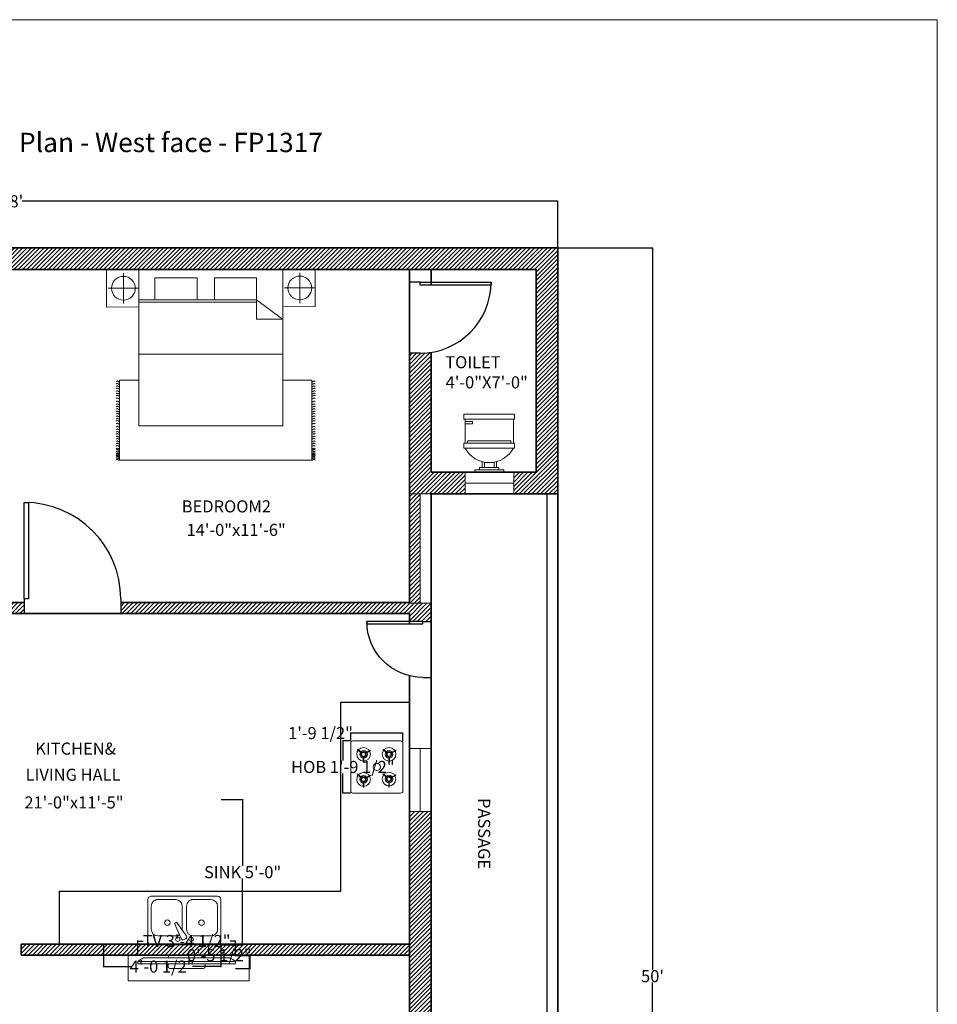
# Model space of a CAD drawing. Units: inches. Extents: x 2202345 to 2203065, y -970921 to -970107.
# Tile 5 of 5: x 2202685 to 2203065, y -970515 to -970107. Entities that reach past the tile are written whole.
import ezdxf

# ---------------------------------------------------------------- set-up
doc = ezdxf.new("R2010")
doc.units = ezdxf.units.IN
doc.header["$MEASUREMENT"] = 0
doc.linetypes.add('HIDDEN', pattern=[0.375, 0.25, -0.125])
doc.layers.get('0').update_dxf_attribs({"color": 13})
for name, color, linetype, lineweight in [('A-ANNO-DIMS', 2, 'Continuous', 18), ('A-ANNO-TEXT', 7, 'Continuous', 25), ('A-ANNO-TTLB', 7, 'HIDDEN', 18), ('A-AREA-IDEN', 7, 'Continuous', 18), ('A-EQPM', 8, 'Continuous', 18), ('A-FLOR-CASE', 252, 'Continuous', 25), ('A-WALL-PATT', 8, 'Continuous', 13), ('C-PROP', 7, 'Continuous', 25), ('doors', 252, 'Continuous', 25), ('furniture', 250, 'Continuous', 18), ('PLUMBING FIXTURES', 8, 'Continuous', 18), ('walls', 252, 'Continuous', 35), ('windows', 173, 'Continuous', 18)]:
    doc.layers.add(name, color=color, linetype=linetype, lineweight=lineweight)
doc.styles.add('ATT', font='TXT')
doc.styles.get("Standard").update_dxf_attribs({"font": 'arial.ttf'})
doc.dimstyles.get("Standard").update_dxf_attribs({"dimtxt": 5, "dimasz": 0.18, "dimexe": 0.18, "dimexo": 0.0625, "dimgap": 0.09, "dimtad": 0, "dimtih": 1, "dimtoh": 1, "dimzin": 0, "dimdsep": 46, "dimlunit": 3, "dimtxsty": 'Standard', "dimcen": 0.09, "dimadec": 0, "dimazin": 0, "dimtfac": 1, "dimtofl": 0, "dimtmove": 0, "dimatfit": 3, "dimfxl": 1, "dimtolj": 1, "dimtzin": 0, "dimarcsym": 0})
pattern_1 = [(45, (0, 0), (-0.8838834765, 0.8838834765), [])]

# ---------------------------------------------------------------- blocks, each defined once
blk = doc.blocks.new('4bstove')
at = {"layer": 'furniture'}
for p, q in [((1452.73, 1446.21), (1452.73, 1448.61)), ((1452.98, 1446.22), (1452.98, 1448.61)), ((1464.44, 1446.34), (1464.44, 1448.73)), ((1464.69, 1446.34), (1464.69, 1448.73)), ((1451.74, 1444.45), (1449.67, 1443.25)), ((1451.87, 1444.23), (1449.79, 1443.04)), ((1453.75, 1444.08), (1455.58, 1442.54)), ((1453.91, 1444.27), (1455.74, 1442.73)), ((1463.45, 1444.58), (1461.38, 1443.38)), ((1463.57, 1444.36), (1461.5, 1443.17)), ((1465.46, 1444.21), (1467.29, 1442.67)), ((1465.62, 1444.4), (1467.45, 1442.86)), ((1452.69, 1434.81), (1452.69, 1437.2)), ((1452.94, 1434.81), (1452.94, 1437.2)), ((1464.44, 1434.81), (1464.44, 1437.2)), ((1464.69, 1434.81), (1464.69, 1437.2)), ((1451.7, 1433.04), (1449.63, 1431.85)), ((1451.82, 1432.83), (1449.75, 1431.63)), ((1453.71, 1432.67), (1455.54, 1431.13)), ((1453.87, 1432.86), (1455.7, 1431.33)), ((1463.45, 1433.04), (1461.38, 1431.85)), ((1463.57, 1432.83), (1461.5, 1431.63)), ((1465.46, 1432.67), (1467.29, 1431.13)), ((1465.62, 1432.86), (1467.45, 1431.33))]:
    blk.add_line(p, q, dxfattribs=at)
for points in [[(1447.5, 1427.38), (1469.5, 1427.38, 0.414214), (1470.5, 1428.38), (1470.5, 1450.38, 0.414214), (1469.5, 1451.38), (1447.5, 1451.38, 0.414214), (1446.5, 1450.38), (1446.5, 1428.38, 0.414214)], [(1453.75, 1444.97, 1), (1452, 1444.97, 1)], [(1465.46, 1445.1, 1), (1463.71, 1445.1, 1)], [(1453.71, 1433.56, 1), (1451.96, 1433.56, 1)], [(1465.46, 1433.56, 1), (1463.71, 1433.56, 1)]]:
    blk.add_lwpolyline(points, format="xyb", close=True, dxfattribs=at)
for points in [[(1454.12, 1444.97, 1), (1451.62, 1444.97, 1), (1454.12, 1444.97, 1)], [(1465.83, 1445.1, 1), (1463.33, 1445.1, 1), (1465.83, 1445.1, 1)], [(1454.08, 1433.56, 1), (1451.58, 1433.56, 1), (1454.08, 1433.56, 1)], [(1465.83, 1433.56, 1), (1463.33, 1433.56, 1), (1465.83, 1433.56, 1)]]:
    blk.add_lwpolyline(points, format="xyb", dxfattribs=at)
for centre, radius in [((1452.87, 1444.97), 3.14), ((1452.87, 1444.97), 1.75), ((1464.58, 1445.1), 3.14), ((1464.58, 1445.1), 1.75), ((1452.83, 1433.56), 3.14), ((1458.5, 1439.38), 1.67), ((1464.58, 1433.56), 3.14), ((1452.83, 1433.56), 1.75), ((1464.58, 1433.56), 1.75)]:
    blk.add_circle(centre, radius, dxfattribs=at)
for centre, start, end in [((1452.87, 1444.97), 88.2645, 92.2039), ((1464.58, 1445.1), 88.2645, 92.2039), ((1452.87, 1444.97), 208.188, 212.1274), ((1452.87, 1444.97), 318.1018, 322.0412), ((1464.58, 1445.1), 208.188, 212.1274), ((1464.58, 1445.1), 318.1018, 322.0412), ((1452.83, 1433.56), 88.2645, 92.2039), ((1464.58, 1433.56), 88.2645, 92.2039)]:
    blk.add_arc(centre, 3.64, start, end, dxfattribs=at)
blk = doc.blocks.new('15PSNK10')
at = {"color": 0, "linetype": 'ByBlock'}
for p, q in [((0, 15), (0, -15)), ((20.5, 16.5), (1.5, 16.5)), ((7, 15), (17.5, 15)), ((22, -15), (22, 15)), ((4, 4), (4, 12)), ((20.5, 12), (20.5, 4)), ((2.37, -0.1), (2.77, 0.6)), ((10.18, -3.57), (4.27, 0.87)), ((17.5, 1), (7, 1)), ((2.88, -1.54), (9.68, -4.43)), ((4, -12), (4, -4)), ((7.04, -1), (17.5, -1)), ((9.68, -4.43), (10.18, -3.57)), ((20.5, -4), (20.5, -12)), ((1.5, -16.5), (20.5, -16.5)), ((17.5, -15), (7, -15))]:
    blk.add_line(p, q, dxfattribs=at)
for centre, radius in [((10, 7.75), 1.25), ((2.5, 3), 1), ((2.5, -3), 1), ((10, -7.75), 1.25)]:
    blk.add_circle(centre, radius, dxfattribs=at)
for centre, radius, start, end in [((1.5, 15), 1.5, 90, 180), ((7, 12), 3, 90, 180), ((17.5, 12), 3, 0, 90), ((20.5, 15), 1.5, 0, 90), ((3.63, 0.1), 1, 50.5377, 150), ((7, 4), 3, 180, 270), ((17.5, 4), 3, 270, 0), ((3.23, -0.6), 1, 150, 249.4623), ((7, -4), 3, 146.607, 180), ((17.5, -4), 3, 0, 90), ((7, -12), 3, 180, 270), ((17.5, -12), 3, 270, 0), ((1.5, -15), 1.5, 180, 270), ((20.5, -15), 1.5, 270, 0)]:
    blk.add_arc(centre, radius, start, end, dxfattribs=at)
at = {"color": 0, "linetype": 'ByBlock', "style": 'ATT'}
for tag, p, flags in [('ITEM', (0, -26), 3), ('ROOM_NUMBER', (0, -35), 1)]:
    blk.add_attdef(tag, p, '', height=6, dxfattribs=dict(at, flags=flags))
blk = doc.blocks.new('PLASMA-LARGE')
at = {"layer": 'furniture'}
for p, q in [((-7.26, 0), (7.26, 0)), ((-21, -2.5), (21, -2.5)), ((-21, -2.5), (-21, -3.5)), ((-21, -3.5), (21, -3.5)), ((-18.61, -1), (18.61, -1)), ((-8, -1), (-8, -0.74)), ((-8, -3.5), (-8, -4.76)), ((8, -1), (8, -0.74)), ((8, -3.5), (8, -4.76)), ((21, -2.5), (21, -3.5)), ((-7.26, -5.5), (7.26, -5.5))]:
    blk.add_line(p, q, dxfattribs=at)
for centre, radius, start, end in [((-7.26, -0.74), 0.744, 90, 180), ((7.26, -0.74), 0.744, 0, 90), ((-13.97, -11.05), 11.07, 114.7602, 129.4175), ((13.97, -11.05), 11.07, 50.5825, 65.2398), ((-7.26, -4.76), 0.744, 180, 270), ((7.26, -4.76), 0.744, 270, 0)]:
    blk.add_arc(centre, radius, start, end, dxfattribs=at)
blk = doc.blocks.new('CARPET')
at = {"layer": 'furniture'}
for p, q in [((-51.53, -98.11), (-51.53, -55.12)), ((-51.53, -55.12), (-41.27, -55.12)), ((36, -55.12), (51.55, -55.12)), ((51.55, -55.12), (51.55, -98.11)), ((51.55, -98.11), (-51.53, -98.11))]:
    blk.add_line(p, q, dxfattribs=at)
for points, knots in [([(-53.37, -55.99), (-53.22, -55.8), (-52.9, -55.41), (-52.34, -55.8), (-51.89, -56.08), (-51.65, -55.91), (-51.53, -55.83)], [0, 0, 0, 0, 0.653278, 1.290138, 1.740457, 2.114451, 2.114451, 2.114451, 2.114451]), ([(-53.37, -57.26), (-53.22, -57.07), (-52.9, -56.67), (-52.34, -57.07), (-51.89, -57.35), (-51.65, -57.17), (-51.53, -57.1)], [0, 0, 0, 0, 0.653278, 1.290138, 1.740457, 2.114451, 2.114451, 2.114451, 2.114451]), ([(53.37, -55.99), (53.22, -55.8), (52.9, -55.41), (52.34, -55.8), (51.89, -56.08), (51.65, -55.91), (51.53, -55.83)], [0, 0, 0, 0, 0.653278, 1.290138, 1.740457, 2.114451, 2.114451, 2.114451, 2.114451]), ([(53.37, -57.26), (53.22, -57.07), (52.9, -56.67), (52.34, -57.07), (51.89, -57.35), (51.65, -57.17), (51.53, -57.1)], [0, 0, 0, 0, 0.653278, 1.290138, 1.740457, 2.114451, 2.114451, 2.114451, 2.114451]), ([(-53.37, -58.59), (-53.22, -58.4), (-52.9, -58.01), (-52.34, -58.4), (-51.89, -58.68), (-51.65, -58.5), (-51.53, -58.43)], [0, 0, 0, 0, 0.653278, 1.290138, 1.740457, 2.114451, 2.114451, 2.114451, 2.114451]), ([(-53.37, -59.78), (-53.22, -59.58), (-52.9, -59.19), (-52.34, -59.58), (-51.89, -59.86), (-51.65, -59.69), (-51.53, -59.61)], [0, 0, 0, 0, 0.653278, 1.290138, 1.740457, 2.114451, 2.114451, 2.114451, 2.114451]), ([(-53.37, -61.22), (-53.22, -61.02), (-52.9, -60.63), (-52.34, -61.02), (-51.89, -61.3), (-51.65, -61.13), (-51.53, -61.05)], [0, 0, 0, 0, 0.653278, 1.290138, 1.740457, 2.114451, 2.114451, 2.114451, 2.114451]), ([(-53.37, -62.44), (-53.22, -62.25), (-52.9, -61.86), (-52.34, -62.25), (-51.89, -62.53), (-51.65, -62.36), (-51.53, -62.28)], [0, 0, 0, 0, 0.653278, 1.290138, 1.740457, 2.114451, 2.114451, 2.114451, 2.114451]), ([(-53.37, -63.63), (-53.22, -63.43), (-52.9, -63.04), (-52.34, -63.43), (-51.89, -63.72), (-51.65, -63.54), (-51.53, -63.46)], [0, 0, 0, 0, 0.653278, 1.290138, 1.740457, 2.114451, 2.114451, 2.114451, 2.114451]), ([(53.37, -58.59), (53.22, -58.4), (52.9, -58.01), (52.34, -58.4), (51.89, -58.68), (51.65, -58.5), (51.53, -58.43)], [0, 0, 0, 0, 0.653278, 1.290138, 1.740457, 2.114451, 2.114451, 2.114451, 2.114451]), ([(53.37, -59.78), (53.22, -59.58), (52.9, -59.19), (52.34, -59.58), (51.89, -59.86), (51.65, -59.69), (51.53, -59.61)], [0, 0, 0, 0, 0.653278, 1.290138, 1.740457, 2.114451, 2.114451, 2.114451, 2.114451]), ([(53.37, -61.22), (53.22, -61.02), (52.9, -60.63), (52.34, -61.02), (51.89, -61.3), (51.65, -61.13), (51.53, -61.05)], [0, 0, 0, 0, 0.653278, 1.290138, 1.740457, 2.114451, 2.114451, 2.114451, 2.114451]), ([(53.37, -62.44), (53.22, -62.25), (52.9, -61.86), (52.34, -62.25), (51.89, -62.53), (51.65, -62.36), (51.53, -62.28)], [0, 0, 0, 0, 0.653278, 1.290138, 1.740457, 2.114451, 2.114451, 2.114451, 2.114451]), ([(53.37, -63.63), (53.22, -63.43), (52.9, -63.04), (52.34, -63.43), (51.89, -63.72), (51.65, -63.54), (51.53, -63.46)], [0, 0, 0, 0, 0.653278, 1.290138, 1.740457, 2.114451, 2.114451, 2.114451, 2.114451]), ([(-53.37, -65.07), (-53.22, -64.87), (-52.9, -64.48), (-52.34, -64.87), (-51.89, -65.15), (-51.65, -64.98), (-51.53, -64.9)], [0, 0, 0, 0, 0.653278, 1.290138, 1.740457, 2.114451, 2.114451, 2.114451, 2.114451]), ([(-53.37, -66.76), (-53.22, -66.56), (-52.9, -66.17), (-52.34, -66.56), (-51.89, -66.84), (-51.65, -66.67), (-51.53, -66.59)], [0, 0, 0, 0, 0.653278, 1.290138, 1.740457, 2.114451, 2.114451, 2.114451, 2.114451]), ([(-53.37, -68.2), (-53.22, -68), (-52.9, -67.61), (-52.34, -68), (-51.89, -68.28), (-51.65, -68.11), (-51.53, -68.03)], [0, 0, 0, 0, 0.653278, 1.290138, 1.740457, 2.114451, 2.114451, 2.114451, 2.114451]), ([(53.37, -65.07), (53.22, -64.87), (52.9, -64.48), (52.34, -64.87), (51.89, -65.15), (51.65, -64.98), (51.53, -64.9)], [0, 0, 0, 0, 0.653278, 1.290138, 1.740457, 2.114451, 2.114451, 2.114451, 2.114451]), ([(53.37, -66.76), (53.22, -66.56), (52.9, -66.17), (52.34, -66.56), (51.89, -66.84), (51.65, -66.67), (51.53, -66.59)], [0, 0, 0, 0, 0.653278, 1.290138, 1.740457, 2.114451, 2.114451, 2.114451, 2.114451]), ([(53.37, -68.2), (53.22, -68), (52.9, -67.61), (52.34, -68), (51.89, -68.28), (51.65, -68.11), (51.53, -68.03)], [0, 0, 0, 0, 0.653278, 1.290138, 1.740457, 2.114451, 2.114451, 2.114451, 2.114451]), ([(-53.37, -69.53), (-53.22, -69.33), (-52.9, -68.94), (-52.34, -69.33), (-51.89, -69.61), (-51.65, -69.44), (-51.53, -69.36)], [0, 0, 0, 0, 0.653278, 1.290138, 1.740457, 2.114451, 2.114451, 2.114451, 2.114451]), ([(-53.37, -70.79), (-53.22, -70.6), (-52.9, -70.21), (-52.34, -70.6), (-51.89, -70.88), (-51.65, -70.7), (-51.53, -70.63)], [0, 0, 0, 0, 0.653278, 1.290138, 1.740457, 2.114451, 2.114451, 2.114451, 2.114451]), ([(-53.37, -72.12), (-53.22, -71.93), (-52.9, -71.54), (-52.34, -71.93), (-51.89, -72.21), (-51.65, -72.04), (-51.53, -71.96)], [0, 0, 0, 0, 0.653278, 1.290138, 1.740457, 2.114451, 2.114451, 2.114451, 2.114451]), ([(-53.37, -73.31), (-53.22, -73.11), (-52.9, -72.72), (-52.34, -73.11), (-51.89, -73.4), (-51.65, -73.22), (-51.53, -73.14)], [0, 0, 0, 0, 0.653278, 1.290138, 1.740457, 2.114451, 2.114451, 2.114451, 2.114451]), ([(53.37, -69.53), (53.22, -69.33), (52.9, -68.94), (52.34, -69.33), (51.89, -69.61), (51.65, -69.44), (51.53, -69.36)], [0, 0, 0, 0, 0.653278, 1.290138, 1.740457, 2.114451, 2.114451, 2.114451, 2.114451]), ([(53.37, -70.79), (53.22, -70.6), (52.9, -70.21), (52.34, -70.6), (51.89, -70.88), (51.65, -70.7), (51.53, -70.63)], [0, 0, 0, 0, 0.653278, 1.290138, 1.740457, 2.114451, 2.114451, 2.114451, 2.114451]), ([(53.37, -72.12), (53.22, -71.93), (52.9, -71.54), (52.34, -71.93), (51.89, -72.21), (51.65, -72.04), (51.53, -71.96)], [0, 0, 0, 0, 0.653278, 1.290138, 1.740457, 2.114451, 2.114451, 2.114451, 2.114451]), ([(53.37, -73.31), (53.22, -73.11), (52.9, -72.72), (52.34, -73.11), (51.89, -73.4), (51.65, -73.22), (51.53, -73.14)], [0, 0, 0, 0, 0.653278, 1.290138, 1.740457, 2.114451, 2.114451, 2.114451, 2.114451]), ([(-53.37, -74.75), (-53.22, -74.55), (-52.9, -74.16), (-52.34, -74.55), (-51.89, -74.83), (-51.65, -74.66), (-51.53, -74.58)], [0, 0, 0, 0, 0.653278, 1.290138, 1.740457, 2.114451, 2.114451, 2.114451, 2.114451]), ([(-53.37, -75.98), (-53.22, -75.78), (-52.9, -75.39), (-52.34, -75.78), (-51.89, -76.06), (-51.65, -75.89), (-51.53, -75.81)], [0, 0, 0, 0, 0.653278, 1.290138, 1.740457, 2.114451, 2.114451, 2.114451, 2.114451]), ([(-53.37, -77.16), (-53.22, -76.96), (-52.9, -76.57), (-52.34, -76.96), (-51.89, -77.25), (-51.65, -77.07), (-51.53, -76.99)], [0, 0, 0, 0, 0.653278, 1.290138, 1.740457, 2.114451, 2.114451, 2.114451, 2.114451]), ([(-53.37, -78.6), (-53.22, -78.4), (-52.9, -78.01), (-52.34, -78.4), (-51.89, -78.68), (-51.65, -78.51), (-51.53, -78.43)], [0, 0, 0, 0, 0.653278, 1.290138, 1.740457, 2.114451, 2.114451, 2.114451, 2.114451]), ([(53.37, -74.75), (53.22, -74.55), (52.9, -74.16), (52.34, -74.55), (51.89, -74.83), (51.65, -74.66), (51.53, -74.58)], [0, 0, 0, 0, 0.653278, 1.290138, 1.740457, 2.114451, 2.114451, 2.114451, 2.114451]), ([(53.37, -75.98), (53.22, -75.78), (52.9, -75.39), (52.34, -75.78), (51.89, -76.06), (51.65, -75.89), (51.53, -75.81)], [0, 0, 0, 0, 0.653278, 1.290138, 1.740457, 2.114451, 2.114451, 2.114451, 2.114451]), ([(53.37, -77.16), (53.22, -76.96), (52.9, -76.57), (52.34, -76.96), (51.89, -77.25), (51.65, -77.07), (51.53, -76.99)], [0, 0, 0, 0, 0.653278, 1.290138, 1.740457, 2.114451, 2.114451, 2.114451, 2.114451]), ([(53.37, -78.6), (53.22, -78.4), (52.9, -78.01), (52.34, -78.4), (51.89, -78.68), (51.65, -78.51), (51.53, -78.43)], [0, 0, 0, 0, 0.653278, 1.290138, 1.740457, 2.114451, 2.114451, 2.114451, 2.114451]), ([(-53.37, -80.29), (-53.22, -80.09), (-52.9, -79.7), (-52.34, -80.09), (-51.89, -80.37), (-51.65, -80.2), (-51.53, -80.12)], [0, 0, 0, 0, 0.653278, 1.290138, 1.740457, 2.114451, 2.114451, 2.114451, 2.114451]), ([(-53.37, -81.73), (-53.22, -81.53), (-52.9, -81.14), (-52.34, -81.53), (-51.89, -81.81), (-51.65, -81.64), (-51.53, -81.56)], [0, 0, 0, 0, 0.653278, 1.290138, 1.740457, 2.114451, 2.114451, 2.114451, 2.114451]), ([(-53.37, -83.06), (-53.22, -82.86), (-52.9, -82.47), (-52.34, -82.86), (-51.89, -83.14), (-51.65, -82.97), (-51.53, -82.89)], [0, 0, 0, 0, 0.653278, 1.290138, 1.740457, 2.114451, 2.114451, 2.114451, 2.114451]), ([(-53.37, -84.18), (-53.22, -83.99), (-52.9, -83.6), (-52.34, -83.99), (-51.89, -84.27), (-51.65, -84.09), (-51.53, -84.02)], [0, 0, 0, 0, 0.653278, 1.290138, 1.740457, 2.114451, 2.114451, 2.114451, 2.114451]), ([(53.37, -80.29), (53.22, -80.09), (52.9, -79.7), (52.34, -80.09), (51.89, -80.37), (51.65, -80.2), (51.53, -80.12)], [0, 0, 0, 0, 0.653278, 1.290138, 1.740457, 2.114451, 2.114451, 2.114451, 2.114451]), ([(53.37, -81.73), (53.22, -81.53), (52.9, -81.14), (52.34, -81.53), (51.89, -81.81), (51.65, -81.64), (51.53, -81.56)], [0, 0, 0, 0, 0.653278, 1.290138, 1.740457, 2.114451, 2.114451, 2.114451, 2.114451]), ([(53.37, -83.06), (53.22, -82.86), (52.9, -82.47), (52.34, -82.86), (51.89, -83.14), (51.65, -82.97), (51.53, -82.89)], [0, 0, 0, 0, 0.653278, 1.290138, 1.740457, 2.114451, 2.114451, 2.114451, 2.114451]), ([(53.37, -84.18), (53.22, -83.99), (52.9, -83.6), (52.34, -83.99), (51.89, -84.27), (51.65, -84.09), (51.53, -84.02)], [0, 0, 0, 0, 0.653278, 1.290138, 1.740457, 2.114451, 2.114451, 2.114451, 2.114451]), ([(-53.37, -85.51), (-53.22, -85.32), (-52.9, -84.93), (-52.34, -85.32), (-51.89, -85.6), (-51.65, -85.42), (-51.53, -85.35)], [0, 0, 0, 0, 0.653278, 1.290138, 1.740457, 2.114451, 2.114451, 2.114451, 2.114451]), ([(-53.37, -86.7), (-53.22, -86.5), (-52.9, -86.11), (-52.34, -86.5), (-51.89, -86.78), (-51.65, -86.61), (-51.53, -86.53)], [0, 0, 0, 0, 0.653278, 1.290138, 1.740457, 2.114451, 2.114451, 2.114451, 2.114451]), ([(-53.37, -88.14), (-53.22, -87.94), (-52.9, -87.55), (-52.34, -87.94), (-51.89, -88.22), (-51.65, -88.05), (-51.53, -87.97)], [0, 0, 0, 0, 0.653278, 1.290138, 1.740457, 2.114451, 2.114451, 2.114451, 2.114451]), ([(-53.37, -89.36), (-53.22, -89.17), (-52.9, -88.78), (-52.34, -89.17), (-51.89, -89.45), (-51.65, -89.28), (-51.53, -89.2)], [0, 0, 0, 0, 0.653278, 1.290138, 1.740457, 2.114451, 2.114451, 2.114451, 2.114451]), ([(53.37, -85.51), (53.22, -85.32), (52.9, -84.93), (52.34, -85.32), (51.89, -85.6), (51.65, -85.42), (51.53, -85.35)], [0, 0, 0, 0, 0.653278, 1.290138, 1.740457, 2.114451, 2.114451, 2.114451, 2.114451]), ([(53.37, -86.7), (53.22, -86.5), (52.9, -86.11), (52.34, -86.5), (51.89, -86.78), (51.65, -86.61), (51.53, -86.53)], [0, 0, 0, 0, 0.653278, 1.290138, 1.740457, 2.114451, 2.114451, 2.114451, 2.114451]), ([(53.37, -88.14), (53.22, -87.94), (52.9, -87.55), (52.34, -87.94), (51.89, -88.22), (51.65, -88.05), (51.53, -87.97)], [0, 0, 0, 0, 0.653278, 1.290138, 1.740457, 2.114451, 2.114451, 2.114451, 2.114451]), ([(53.37, -89.36), (53.22, -89.17), (52.9, -88.78), (52.34, -89.17), (51.89, -89.45), (51.65, -89.28), (51.53, -89.2)], [0, 0, 0, 0, 0.653278, 1.290138, 1.740457, 2.114451, 2.114451, 2.114451, 2.114451]), ([(-53.37, -90.55), (-53.22, -90.35), (-52.9, -89.96), (-52.34, -90.35), (-51.89, -90.64), (-51.65, -90.46), (-51.53, -90.38)], [0, 0, 0, 0, 0.653278, 1.290138, 1.740457, 2.114451, 2.114451, 2.114451, 2.114451]), ([(-53.37, -91.99), (-53.22, -91.79), (-52.9, -91.4), (-52.34, -91.79), (-51.89, -92.07), (-51.65, -91.9), (-51.53, -91.82)], [0, 0, 0, 0, 0.653278, 1.290138, 1.740457, 2.114451, 2.114451, 2.114451, 2.114451]), ([(-53.37, -92.69), (-53.22, -92.48), (-52.9, -92.08), (-52.35, -92.49), (-51.89, -92.77), (-51.65, -92.6), (-51.53, -92.52)], [0, 0, 0, 0, 0.663904, 1.307406, 1.757725, 2.131719, 2.131719, 2.131719, 2.131719]), ([(-53.37, -93.61), (-53.22, -93.42), (-52.9, -93.03), (-52.34, -93.42), (-51.89, -93.7), (-51.65, -93.52), (-51.53, -93.45)], [0, 0, 0, 0, 0.653278, 1.290138, 1.740457, 2.114451, 2.114451, 2.114451, 2.114451]), ([(-53.37, -94.55), (-53.22, -94.35), (-52.9, -93.96), (-52.34, -94.35), (-51.89, -94.63), (-51.65, -94.46), (-51.53, -94.38)], [0, 0, 0, 0, 0.653278, 1.290138, 1.740457, 2.114451, 2.114451, 2.114451, 2.114451]), ([(-53.37, -95.05), (-53.22, -94.85), (-52.9, -94.46), (-52.34, -94.85), (-51.89, -95.14), (-51.65, -94.96), (-51.53, -94.88)], [0, 0, 0, 0, 0.653278, 1.290138, 1.740457, 2.114451, 2.114451, 2.114451, 2.114451]), ([(53.37, -90.55), (53.22, -90.35), (52.9, -89.96), (52.34, -90.35), (51.9, -90.63), (51.66, -90.47), (51.55, -90.4)], [0, 0, 0, 0, 0.653278, 1.290138, 1.740457, 2.0926, 2.0926, 2.0926, 2.0926]), ([(53.37, -91.99), (53.22, -91.79), (52.9, -91.4), (52.34, -91.79), (51.9, -92.07), (51.66, -91.91), (51.55, -91.83)], [0, 0, 0, 0, 0.653278, 1.290138, 1.740457, 2.0926, 2.0926, 2.0926, 2.0926]), ([(53.37, -92.69), (53.22, -92.49), (52.9, -92.09), (52.34, -92.49), (51.9, -92.77), (51.66, -92.61), (51.55, -92.53)], [0, 0, 0, 0, 0.656792, 1.295826, 1.746145, 2.098292, 2.098292, 2.098292, 2.098292]), ([(53.37, -93.66), (53.22, -93.46), (52.9, -93.07), (52.34, -93.46), (51.9, -93.74), (51.66, -93.58), (51.55, -93.5)], [0, 0, 0, 0, 0.653278, 1.290138, 1.740457, 2.0926, 2.0926, 2.0926, 2.0926]), ([(53.37, -94.59), (53.22, -94.4), (52.9, -94.01), (52.34, -94.4), (51.9, -94.68), (51.66, -94.51), (51.55, -94.44)], [0, 0, 0, 0, 0.653278, 1.290138, 1.740457, 2.0926, 2.0926, 2.0926, 2.0926]), ([(53.37, -95.1), (53.22, -94.9), (52.9, -94.51), (52.34, -94.9), (51.9, -95.18), (51.66, -95.02), (51.55, -94.94)], [0, 0, 0, 0, 0.653278, 1.290138, 1.740457, 2.0926, 2.0926, 2.0926, 2.0926]), ([(-53.37, -95.73), (-53.22, -95.54), (-52.9, -95.15), (-52.34, -95.54), (-51.89, -95.82), (-51.65, -95.65), (-51.53, -95.57)], [0, 0, 0, 0, 0.653278, 1.290138, 1.740457, 2.114451, 2.114451, 2.114451, 2.114451]), ([(-53.37, -96.38), (-53.22, -96.18), (-52.9, -95.79), (-52.34, -96.18), (-51.89, -96.47), (-51.65, -96.29), (-51.53, -96.21)], [0, 0, 0, 0, 0.653278, 1.290138, 1.740457, 2.114451, 2.114451, 2.114451, 2.114451]), ([(-53.37, -97.17), (-53.22, -96.98), (-52.9, -96.59), (-52.34, -96.98), (-51.89, -97.26), (-51.65, -97.08), (-51.53, -97.01)], [0, 0, 0, 0, 0.653278, 1.290138, 1.740457, 2.114451, 2.114451, 2.114451, 2.114451]), ([(-53.37, -97.99), (-53.22, -97.79), (-52.9, -97.4), (-52.34, -97.79), (-51.89, -98.08), (-51.65, -97.9), (-51.53, -97.82)], [0, 0, 0, 0, 0.653278, 1.290138, 1.740457, 2.114451, 2.114451, 2.114451, 2.114451]), ([(53.37, -95.78), (53.22, -95.58), (52.9, -95.19), (52.34, -95.58), (51.89, -95.86), (51.65, -95.69), (51.53, -95.61)], [0, 0, 0, 0, 0.653278, 1.290138, 1.740457, 2.114451, 2.114451, 2.114451, 2.114451]), ([(53.37, -96.43), (53.22, -96.23), (52.9, -95.84), (52.34, -96.23), (51.89, -96.51), (51.65, -96.34), (51.53, -96.26)], [0, 0, 0, 0, 0.653278, 1.290138, 1.740457, 2.114451, 2.114451, 2.114451, 2.114451]), ([(53.37, -97.22), (53.22, -97.02), (52.9, -96.63), (52.34, -97.02), (51.89, -97.3), (51.65, -97.13), (51.53, -97.05)], [0, 0, 0, 0, 0.653278, 1.290138, 1.740457, 2.114451, 2.114451, 2.114451, 2.114451]), ([(53.37, -97.99), (53.22, -97.79), (52.9, -97.4), (52.34, -97.79), (51.89, -98.08), (51.65, -97.9), (51.53, -97.82)], [0, 0, 0, 0, 0.653278, 1.290138, 1.740457, 2.114451, 2.114451, 2.114451, 2.114451])]:
    blk.add_open_spline(points, degree=3, knots=knots, dxfattribs=at)
blk = doc.blocks.new('A$C58D270C6')
at = {"layer": 'furniture'}
for p, q in [((9.09, 124.13), (9.09, 108.87)), ((1.46, 116.5), (16.73, 116.5)), ((14.97, 94.84), (24.62, 107.92)), ((24.62, 94.93), (24.62, 107.92)), ((42.08, 108), (42.08, 36)), ((14.97, 94.93), (24.62, 94.93)), ((14.97, 94.84), (14.97, 36)), ((16.22, 94.93), (16.22, 36)), ((9.25, 36), (9.25, 20.74)), ((1.62, 28.37), (16.88, 28.37))]:
    blk.add_line(p, q, dxfattribs=at)
for points in [[(18.5, 108), (18.34, 124.13), (-0.16, 124.13), (0, 108)], [(0, 108), (77.91, 108), (77.91, 36), (0, 36)], [(4.09, 94.93), (14.97, 94.93), (14.97, 73.83), (4.09, 73.83)], [(4.09, 65.23), (14.97, 65.23), (14.97, 44.13), (4.09, 44.13)], [(18.65, 19.87), (18.5, 36), (0, 36), (0.16, 19.87)]]:
    blk.add_lwpolyline(points, close=True, dxfattribs=at)
for centre in [(9.09, 116.5), (9.25, 28.37)]:
    blk.add_circle(centre, 5.95, dxfattribs=at)
at = {"layer": 'furniture', "xscale": 0.9312884925094044, "yscale": 0.9312884925094044, "zscale": 0.9312884925094044, "rotation": 90}
blk.add_blockref('CARPET', (3.79, 74.47), dxfattribs=at)
blk = doc.blocks.new('*U12')
for p, q in [((0, 0), (0, -6)), ((40, 0), (40, -6))]:
    blk.add_line(p, q)
blk.add_lwpolyline([(0, 0), (0, 40), (1.75, 40), (1.75, 0)], close=True)
blk.add_arc((0, 0), 40, 0, 90)
blk = doc.blocks.new('*U2')
for p, q in [((-10, 22), (-10, 12)), ((-10, 21), (-7, 21)), ((-7, 21), (-7, 20)), ((10, 12), (10, 22)), ((-7, 20), (-10, 20)), ((9, 13), (-9, 13)), ((-9, 13), (-9, 12)), ((9, 12), (9, 13)), ((10.5, 12), (-10.5, 12)), ((-10.5, 10), (-10.5, 12)), ((10.5, 10), (-10.5, 10)), ((10.5, 12), (10.5, 10)), ((-3, 4.4065), (-3, 2)), ((-2, 2), (-2, 4.1658)), ((2, 4.1658), (2, 2)), ((3, 2), (3, 4.4065)), ((4, 2), (-4, 2)), ((-4, 2), (-4, 1)), ((4, 1), (4, 2))]:
    blk.add_line(p, q)
for points in [[(10.5, 22), (10.5, 24), (-10.5, 24), (-10.5, 22)], [(6, 0), (6, 1), (-6, 1), (-6, 0)]]:
    blk.add_lwpolyline(points, close=True)
blk.add_arc((0, 15.3333), 11.3333, 208.0725, 331.9275)
blk = doc.blocks.new('*D20')
at = {"layer": 'A-ANNO-DIMS', "color": 0, "lineweight": -2, "transparency": 16777216}
for p, q in [((2202455.18, -970201.04), (2202455.18, -970181.68)), ((2202455.36, -970181.86), (2202677.1, -970181.86)), ((2202907.5, -970181.86), (2202685.76, -970181.86)), ((2202907.68, -970201.04), (2202907.68, -970181.68))]:
    blk.add_line(p, q, dxfattribs=at)
at = {"layer": 'A-ANNO-DIMS', "color": 0, "transparency": 16777216}
for points in [[(2202455.36, -970181.83), (2202455.36, -970181.89), (2202455.18, -970181.86)], [(2202907.5, -970181.83), (2202907.5, -970181.89), (2202907.68, -970181.86)]]:
    blk.add_solid(points, dxfattribs=at)
at = {"layer": 'Defpoints', "color": 0, "transparency": 16777216}
for p in [(2202907.68, -970181.86), (2202455.18, -970201.11), (2202907.68, -970201.11)]:
    blk.add_point(p, dxfattribs=at)
at = {"layer": 'A-ANNO-DIMS', "color": 0, "transparency": 16777216, "insert": (2202681.43, -970181.86), "char_height": 5, "attachment_point": 5}
blk.add_mtext("\\A1;38'", dxfattribs=at)
blk = doc.blocks.new('*D21')
at = {"layer": 'A-ANNO-DIMS', "color": 0, "lineweight": -2, "transparency": 16777216}
for p, q in [((2202907.74, -970201.11), (2202947.11, -970201.11)), ((2202946.93, -970201.29), (2202946.93, -970500.21)), ((2202946.93, -970804.43), (2202946.93, -970505.5)), ((2202907.74, -970804.61), (2202947.11, -970804.61))]:
    blk.add_line(p, q, dxfattribs=at)
at = {"layer": 'A-ANNO-DIMS', "color": 0, "transparency": 16777216}
for points in [[(2202946.9, -970201.29), (2202946.96, -970201.29), (2202946.93, -970201.11)], [(2202946.9, -970804.43), (2202946.96, -970804.43), (2202946.93, -970804.61)]]:
    blk.add_solid(points, dxfattribs=at)
at = {"layer": 'Defpoints', "color": 0, "transparency": 16777216}
for p in [(2202907.68, -970201.11), (2202907.68, -970804.61), (2202946.93, -970804.61)]:
    blk.add_point(p, dxfattribs=at)
at = {"layer": 'A-ANNO-DIMS', "color": 0, "transparency": 16777216, "insert": (2202946.93, -970502.86), "char_height": 5, "attachment_point": 5}
blk.add_mtext("\\A1;50'", dxfattribs=at)
blk = doc.blocks.new('*D31')
at = {"layer": 'A-ANNO-DIMS', "color": 0, "lineweight": -2, "transparency": 16777216}
for p, q in [((2202821.8, -970405.4), (2202818.44, -970405.4)), ((2202818.62, -970405.58), (2202818.62, -970413.52)), ((2202818.62, -970426.82), (2202818.62, -970418.88)), ((2202821.8, -970427), (2202818.44, -970427))]:
    blk.add_line(p, q, dxfattribs=at)
at = {"layer": 'A-ANNO-DIMS', "color": 0, "transparency": 16777216}
for points in [[(2202818.59, -970405.58), (2202818.65, -970405.58), (2202818.62, -970405.4)], [(2202818.59, -970426.82), (2202818.65, -970426.82), (2202818.62, -970427)]]:
    blk.add_solid(points, dxfattribs=at)
at = {"layer": 'Defpoints', "color": 0, "transparency": 16777216}
for p in [(2202821.86, -970405.4), (2202818.62, -970427), (2202821.86, -970427)]:
    blk.add_point(p, dxfattribs=at)
at = {"layer": 'A-ANNO-DIMS', "color": 0, "transparency": 16777216, "insert": (2202818.62, -970416.2), "char_height": 5, "attachment_point": 5}
blk.add_mtext('\\A1;HOB 1\'-9 1/2"', dxfattribs=at)
blk = doc.blocks.new('*D32')
at = {"layer": 'A-ANNO-DIMS', "color": 0, "lineweight": -2, "transparency": 16777216}
for p, q in [((2202821.86, -970402.16), (2202821.68, -970402.16)), ((2202821.86, -970405.34), (2202821.86, -970401.98)), ((2202843.28, -970402.16), (2202822.04, -970402.16)), ((2202843.46, -970405.34), (2202843.46, -970401.98))]:
    blk.add_line(p, q, dxfattribs=at)
at = {"layer": 'A-ANNO-DIMS', "color": 0, "transparency": 16777216}
for points in [[(2202822.04, -970402.13), (2202822.04, -970402.19), (2202821.86, -970402.16)], [(2202843.28, -970402.13), (2202843.28, -970402.19), (2202843.46, -970402.16)]]:
    blk.add_solid(points, dxfattribs=at)
at = {"layer": 'Defpoints', "color": 0, "transparency": 16777216}
for p in [(2202821.86, -970402.16), (2202821.86, -970405.4), (2202843.46, -970405.4)]:
    blk.add_point(p, dxfattribs=at)
at = {"layer": 'A-ANNO-DIMS', "color": 0, "transparency": 16777216, "insert": (2202809.36, -970402.16), "char_height": 5, "attachment_point": 5}
blk.add_mtext('\\A1;1\'-9 1/2"', dxfattribs=at)
blk = doc.blocks.new('*D33')
at = {"layer": 'A-ANNO-DIMS', "color": 0, "lineweight": -2, "transparency": 16777216}
for p, q in [((2202768.12, -970429.7), (2202777.26, -970429.7)), ((2202777.08, -970429.88), (2202777.08, -970457.11)), ((2202777.08, -970489.68), (2202777.08, -970462.46)), ((2202768.12, -970489.86), (2202777.26, -970489.86))]:
    blk.add_line(p, q, dxfattribs=at)
at = {"layer": 'A-ANNO-DIMS', "color": 0, "transparency": 16777216}
for points in [[(2202777.05, -970429.88), (2202777.11, -970429.88), (2202777.08, -970429.7)], [(2202777.05, -970489.68), (2202777.11, -970489.68), (2202777.08, -970489.86)]]:
    blk.add_solid(points, dxfattribs=at)
at = {"layer": 'Defpoints', "color": 0, "transparency": 16777216}
for p in [(2202768.06, -970429.7), (2202777.08, -970429.7), (2202768.06, -970489.86)]:
    blk.add_point(p, dxfattribs=at)
at = {"layer": 'A-ANNO-DIMS', "color": 0, "transparency": 16777216, "insert": (2202777.08, -970459.78), "char_height": 5, "attachment_point": 5}
blk.add_mtext('\\A1;SINK 5\'-0"', dxfattribs=at)
blk = doc.blocks.new('*D34')
at = {"layer": 'A-ANNO-DIMS', "color": 0, "lineweight": -2, "transparency": 16777216}
for p, q in [((2202719.36, -970489.93), (2202719.36, -970499.07)), ((2202768.06, -970489.93), (2202768.06, -970499.07)), ((2202719.54, -970498.89), (2202731.05, -970498.89)), ((2202767.88, -970498.89), (2202756.37, -970498.89))]:
    blk.add_line(p, q, dxfattribs=at)
at = {"layer": 'A-ANNO-DIMS', "color": 0, "transparency": 16777216}
for points in [[(2202719.54, -970498.86), (2202719.54, -970498.92), (2202719.36, -970498.89)], [(2202767.88, -970498.86), (2202767.88, -970498.92), (2202768.06, -970498.89)]]:
    blk.add_solid(points, dxfattribs=at)
at = {"layer": 'Defpoints', "color": 0, "transparency": 16777216}
for p in [(2202719.36, -970489.86), (2202768.06, -970489.86), (2202768.06, -970498.89)]:
    blk.add_point(p, dxfattribs=at)
at = {"layer": 'A-ANNO-DIMS', "color": 0, "transparency": 16777216, "insert": (2202743.71, -970498.89), "char_height": 5, "attachment_point": 5}
blk.add_mtext('\\A1;4\'-0 1/2"', dxfattribs=at)
blk = doc.blocks.new('*D37')
at = {"layer": 'A-ANNO-DIMS', "color": 0, "lineweight": -2, "transparency": 16777216}
for p, q in [((2202733.64, -970494.3), (2202733.64, -970488.12)), ((2202733.82, -970488.3), (2202735.81, -970488.3)), ((2202773.9, -970488.3), (2202771.92, -970488.3)), ((2202774.08, -970494.3), (2202774.08, -970488.12))]:
    blk.add_line(p, q, dxfattribs=at)
at = {"layer": 'A-ANNO-DIMS', "color": 0, "transparency": 16777216}
for points in [[(2202733.82, -970488.27), (2202733.82, -970488.33), (2202733.64, -970488.3)], [(2202773.9, -970488.27), (2202773.9, -970488.33), (2202774.08, -970488.3)]]:
    blk.add_solid(points, dxfattribs=at)
at = {"layer": 'Defpoints', "color": 0, "transparency": 16777216}
for p in [(2202733.64, -970488.3), (2202733.64, -970494.37), (2202774.08, -970494.36)]:
    blk.add_point(p, dxfattribs=at)
at = {"layer": 'A-ANNO-DIMS', "color": 0, "transparency": 16777216, "insert": (2202753.86, -970488.3), "char_height": 5, "attachment_point": 5}
blk.add_mtext('\\A1;TV 3\'-4 1/2"', dxfattribs=at)
blk = doc.blocks.new('*D38')
at = {"layer": 'A-ANNO-DIMS', "color": 0, "lineweight": -2, "transparency": 16777216}
for p, q in [((2202774.15, -970494.36), (2202780.33, -970494.36)), ((2202780.15, -970494.18), (2202779.97, -970494.18)), ((2202780.15, -970494.36), (2202780.15, -970494.18)), ((2202780.15, -970499.48), (2202780.15, -970494.54)), ((2202774.15, -970499.66), (2202780.33, -970499.66))]:
    blk.add_line(p, q, dxfattribs=at)
at = {"layer": 'A-ANNO-DIMS', "color": 0, "transparency": 16777216}
for points in [[(2202780.18, -970494.54), (2202780.12, -970494.54), (2202780.15, -970494.36)], [(2202780.18, -970499.48), (2202780.12, -970499.48), (2202780.15, -970499.66)]]:
    blk.add_solid(points, dxfattribs=at)
at = {"layer": 'Defpoints', "color": 0, "transparency": 16777216}
for p in [(2202774.08, -970494.36), (2202780.15, -970494.36), (2202774.08, -970499.66)]:
    blk.add_point(p, dxfattribs=at)
at = {"layer": 'A-ANNO-DIMS', "color": 0, "transparency": 16777216, "insert": (2202767.41, -970494.18), "char_height": 5, "attachment_point": 5}
blk.add_mtext('\\A1;0\'-5 1/2"', dxfattribs=at)

msp = doc.modelspace()

# ---------------------------------------------------------------- hatches: boundary and pattern name
at = {"layer": 'A-WALL-PATT'}
h = msp.add_hatch(dxfattribs=at)
h.set_pattern_fill('ANSI31', color=256, scale=10)
h.set_pattern_definition(pattern_1)
h.paths.add_polyline_path([(2202648.182, -970512.768), (2202644.707, -970512.768, -0.0110733), (2202643.682, -970512.746), (2202643.682, -970601.606), (2202609.913, -970601.606), (2202609.913, -970610.606), (2202643.682, -970610.606), (2202643.682, -970619.168), (2202647.677, -970619.168, -0.0047326), (2202648.182, -970619.173)])
h.paths.add_polyline_path([(2202643.682, -970610.606), (2202636.037, -970610.606), (2202636.037, -970659.106), (2202643.682, -970659.106)])
h.paths.add_polyline_path([(2202722.39, -970654.606), (2202722.39, -970650.106), (2202648.182, -970650.106), (2202648.182, -970645.806), (2202647.677, -970645.806), (2202643.682, -970645.806), (2202643.682, -970659.106), (2202722.39, -970659.106)])
h.paths.add_polyline_path([(2202846.182, -970650.106), (2202798.148, -970650.106), (2202798.148, -970659.106), (2202846.182, -970659.106)])
h.paths.add_polyline_path([(2202855.182, -970619.995), (2202846.182, -970619.995), (2202846.182, -970682.124), (2202855.182, -970682.124)])
h.paths.add_polyline_path([(2202855.182, -970434.646), (2202846.182, -970434.646), (2202846.182, -970545.038), (2202855.182, -970545.038)])
h.paths.add_polyline_path([(2202903.182, -970745.106), (2202855.182, -970745.106), (2202855.182, -970729.208), (2202846.182, -970729.208), (2202846.182, -970745.106), (2202725.91, -970745.106), (2202725.91, -970754.106), (2202903.182, -970754.106)])
h.paths.add_polyline_path([(2202846.182, -970489.606), (2202767.486, -970489.606, -0.1570508), (2202766.685, -970489.864), (2202739.229, -970489.864, -0.1570508), (2202738.428, -970489.606), (2202685.343, -970489.606), (2202685.343, -970494.106), (2202846.182, -970494.106)])
h.paths.add_polyline_path([(2202648.182, -970477.106), (2202594.182, -970477.106), (2202594.182, -970352.606), (2202624.243, -970352.606), (2202624.243, -970348.106), (2202575.482, -970348.106), (2202575.482, -970352.606), (2202589.682, -970352.606), (2202589.682, -970412.606), (2202505.682, -970412.606), (2202505.682, -970417.106), (2202589.682, -970417.106), (2202589.682, -970477.106), (2202580.925, -970477.106), (2202580.925, -970481.606), (2202643.682, -970481.606), (2202643.682, -970489.606), (2202644.707, -970489.606), (2202648.182, -970489.606)])
h.paths.add_polyline_path([(2202505.682, -970305.515), (2202496.682, -970305.515), (2202496.682, -970378.877), (2202501.298, -970378.877), (2202505.682, -970378.877)])
h.paths.add_polyline_path([(2202540.998, -970348.106), (2202505.682, -970348.106), (2202505.682, -970352.606), (2202540.998, -970352.606)], flags=17)
h.paths.add_polyline_path([(2202505.682, -970452.918), (2202496.682, -970452.918), (2202496.682, -970516.267), (2202505.682, -970516.267)])
h.paths.add_polyline_path([(2202505.682, -970210.106), (2202898.682, -970210.106), (2202898.682, -970294.106), (2202889.459, -970294.106), (2202889.459, -970303.106), (2202907.682, -970303.106), (2202907.682, -970201.106), (2202496.682, -970201.106), (2202496.682, -970242.728), (2202505.682, -970242.728)])
h.paths.add_polyline_path([(2202678.182, -970210.106), (2202673.682, -970210.106), (2202673.682, -970348.106), (2202664.243, -970348.106), (2202664.243, -970352.606), (2202686.569, -970352.606), (2202686.569, -970348.106), (2202678.182, -970348.106)])
h.paths.add_polyline_path([(2202752.572, -970321.843), (2202794.204, -970321.843), (2202794.204, -970314.185), (2202752.572, -970314.185)], flags=9)
h.paths.add_polyline_path([(2202750.562, -970312.127), (2202793.125, -970312.127), (2202793.125, -970304.366), (2202750.562, -970304.366)], flags=9)
h = msp.add_hatch(dxfattribs=at)
h.set_pattern_fill('ANSI31', color=256, scale=10)
h.set_pattern_definition(pattern_1)
h.paths.add_polyline_path([(2202855.182, -970348.334), (2202850.682, -970348.334), (2202850.682, -970303.106), (2202846.182, -970303.106), (2202846.182, -970348.106), (2202726.569, -970348.106), (2202726.569, -970352.606), (2202846.182, -970352.606), (2202846.182, -970355.92), (2202851.707, -970355.92), (2202855.182, -970355.92)])
h.paths.add_polyline_path([(2202855.182, -970244.428, -0.0391226), (2202850.597, -970244.787), (2202846.182, -970244.787), (2202846.182, -970303.106), (2202850.682, -970303.106), (2202855.182, -970303.106), (2202869.292, -970303.106), (2202869.292, -970298.606), (2202869.292, -970294.106), (2202855.182, -970294.106)])

# ---------------------------------------------------------------- linework, layer by layer
at = {"layer": 'A-ANNO-TTLB'}
for p, q in [((2203064.943, -970106.63), (2202344.52, -970106.63)), ((2203064.943, -970920.555), (2203064.943, -970106.63))]:
    msp.add_line(p, q, dxfattribs=at)
at = {"layer": 'A-FLOR-CASE'}
for p, q in [((2202817.72, -970467.652), (2202817.72, -970389.42)), ((2202817.72, -970389.42), (2202846.182, -970389.42)), ((2202701.216, -970489.606), (2202701.216, -970467.652)), ((2202701.216, -970467.652), (2202817.72, -970467.652))]:
    msp.add_line(p, q, dxfattribs=at)
at = {"layer": 'C-PROP'}
msp.add_line((2202903.182, -970303.106), (2202903.182, -970800.106), dxfattribs=at)
at = {"layer": 'furniture'}
msp.add_lwpolyline([(2202779.738, -970504.736), (2202729.591, -970504.736), (2202729.591, -970494.364), (2202779.738, -970494.364)], close=True, dxfattribs=at)
at = {"layer": 'walls'}
for p, q in [((2202496.682, -970201.106), (2202907.682, -970201.106)), ((2202907.682, -970201.106), (2202907.682, -970804.606)), ((2202505.682, -970210.106), (2202898.682, -970210.106)), ((2202846.182, -970210.106), (2202846.182, -970348.106)), ((2202855.182, -970210.106), (2202855.182, -970216.642)), ((2202898.682, -970210.106), (2202898.682, -970294.106)), ((2202855.182, -970244.428), (2202855.182, -970294.106)), ((2202855.182, -970294.106), (2202898.682, -970294.106)), ((2202855.182, -970303.106), (2202907.682, -970303.106)), ((2202855.182, -970303.106), (2202855.182, -970745.106)), ((2202678.182, -970348.106), (2202686.569, -970348.106)), ((2202726.569, -970348.106), (2202846.182, -970348.106)), ((2202594.182, -970352.606), (2202846.182, -970352.606)), ((2202846.182, -970352.606), (2202846.182, -970356.933)), ((2202846.182, -970378.414), (2202846.182, -970745.106)), ((2202685.343, -970489.606), (2202846.182, -970489.606)), ((2202685.343, -970489.606), (2202685.343, -970494.106)), ((2202685.343, -970494.106), (2202846.182, -970494.106))]:
    msp.add_line(p, q, dxfattribs=at)
at = {"layer": 'windows'}
for p, q in [((2202869.292, -970294.106), (2202869.292, -970303.106)), ((2202889.459, -970298.606), (2202889.459, -970294.106)), ((2202889.459, -970294.106), (2202889.459, -970303.106)), ((2202869.292, -970303.106), (2202869.292, -970298.606)), ((2202869.292, -970298.606), (2202889.459, -970298.606)), ((2202855.182, -970303.106), (2202846.182, -970303.106)), ((2202846.182, -970303.106), (2202850.682, -970303.106)), ((2202850.682, -970303.106), (2202850.682, -970348.334)), ((2202850.682, -970348.334), (2202846.182, -970348.334)), ((2202846.182, -970348.334), (2202855.182, -970348.334)), ((2202846.182, -970408.577), (2202855.182, -970408.577)), ((2202855.182, -970408.577), (2202850.682, -970408.577)), ((2202850.682, -970408.577), (2202850.682, -970434.646)), ((2202850.682, -970434.646), (2202846.182, -970434.646)), ((2202846.182, -970434.646), (2202855.182, -970434.646))]:
    msp.add_line(p, q, dxfattribs=at)

# ---------------------------------------------------------------- block references
at = {"layer": 'A-EQPM'}
for name, p, xscale, yscale, zscale, rotation in [('4bstove', (2204145.316, -969120.757), 0.9, 0.9, 0.9, 180), ('PLASMA-LARGE', (2202753.864, -970494.364), -0.9628364592350681, 0.9628364592350692, 0.9628364592350692, 0.0045102986113932)]:
    msp.add_blockref(name, p, dxfattribs=dict(at, xscale=xscale, yscale=yscale, zscale=zscale, rotation=rotation))
at = {"layer": 'doors'}
for p, xscale, yscale, zscale, rotation in [((2202850.597, -970215.354), 0.7358381503188096, 0.7358381503188096, 0.7358381503188096, 270), ((2202851.707, -970355.92), -0.5790702303642968, 0.5790702303642968, 0.5790702303642968, 90)]:
    msp.add_blockref('*U12', p, dxfattribs=dict(at, xscale=xscale, yscale=yscale, zscale=zscale, rotation=rotation))
msp.add_blockref('*U12', (2202686.569, -970346.606), dxfattribs=at)
at = {"layer": 'furniture', "xscale": 0.8292897843380787, "yscale": 0.8292897843380787, "zscale": 0.8292897843380787, "rotation": 270}
msp.add_blockref('A$C58D270C6', (2202704.149, -970210.234), dxfattribs=at)
at = {"layer": 'PLUMBING FIXTURES'}
msp.add_blockref('*U2', (2202879.279, -970294.106), dxfattribs=at)
at = {"layer": 'PLUMBING FIXTURES', "xscale": -0.9152100227068082, "yscale": 0.9152100227068082, "zscale": 0.9152100227068082, "rotation": 270}
msp.add_blockref('15PSNK10', (2202752.957, -970489.864), dxfattribs=at)

# ---------------------------------------------------------------- texts
at = {"layer": 'A-ANNO-TEXT'}
msp.add_text('38x50 [1900 sq ft ] House Plan - West face - FP1317', height=8, dxfattribs=at).set_placement((2202556.608, -970161.49))
at = {"layer": 'A-AREA-IDEN'}
for s, p in [('TOILET', (2202861.05, -970251.032)), ('4\'-0"X7\'-0"', (2202861.223, -970259.363)), ('BEDROOM2', (2202751.855, -970310.748)), ('14\'-0"x11\'-6"', (2202753.848, -970320.482)), ('KITCHEN&', (2202691.152, -970411.099)), ('LIVING HALL', (2202687.157, -970421.927)), ('21\'-0"x11\'-5"', (2202686.645, -970433.399))]:
    msp.add_text(s, height=5, dxfattribs=at).set_placement(p)
msp.add_text('PASSAGE', height=5, rotation=270, dxfattribs=at).set_placement((2202874.664, -970429.064))

# ---------------------------------------------------------------- dimensions: what is measured, and where the dimension line sits
at = {"layer": 'A-ANNO-DIMS'}
dim = msp.add_linear_dim(base=(2202907.682, -970181.861), p1=(2202455.182, -970201.106), p2=(2202907.682, -970201.106), text="38'", dimstyle='Standard', override={"dimclrd": 0, "dimclre": 0, "dimclrt": 0}, dxfattribs=at)
dim.commit()
dim.dimension.update_dxf_attribs({"geometry": '*D20', "text_midpoint": (2202681.432, -970181.861)})
for base, p1, p2, angle, text, override, picture, middle in [((2202946.927, -970804.606), (2202907.682, -970201.106), (2202907.682, -970804.606), 90, "50'", {"dimclrd": 0, "dimclre": 0, "dimclrt": 0}, '*D21', (2202946.927, -970502.856)), ((2202818.624, -970426.999), (2202821.864, -970405.399), (2202821.864, -970426.999), 270, 'HOB <>', {"dimdec": 1, "dimlfac": 1, "dimrnd": 0, "dimzin": 1, "dimdsep": 46, "dimlunit": 4, "dimfrac": 2}, '*D31', (2202818.624, -970416.199)), ((2202777.083, -970429.699), (2202768.058, -970489.864), (2202768.058, -970429.699), 90, 'SINK <>', {"dimdec": 1, "dimlfac": 1, "dimrnd": 0, "dimzin": 1, "dimdsep": 46, "dimlunit": 4, "dimfrac": 2}, '*D33', (2202777.083, -970459.781)), ((2202733.644, -970488.299), (2202774.083, -970494.362), (2202733.644, -970494.365), 180.00451, 'TV <>', {"dimdec": 1, "dimlfac": 1, "dimrnd": 0, "dimzin": 1, "dimdsep": 46, "dimlunit": 4, "dimfrac": 2}, '*D37', (2202753.863, -970488.298))]:
    dim = msp.add_linear_dim(base=base, p1=p1, p2=p2, angle=angle, text=text, dimstyle='Standard', override=override, dxfattribs=at)
    dim.commit()
    dim.dimension.update_dxf_attribs({"geometry": picture, "text_midpoint": middle})
for base, p1, p2, angle, picture, middle in [((2202821.864, -970402.159), (2202843.464, -970405.399), (2202821.864, -970405.399), 180, '*D32', (2202809.358, -970402.159)), ((2202780.149, -970494.361), (2202774.084, -970499.658), (2202774.083, -970494.362), 90.00451, '*D38', (2202767.408, -970494.181))]:
    dim = msp.add_linear_dim(base=base, p1=p1, p2=p2, angle=angle, dimstyle='Standard', override={"dimdec": 1, "dimlfac": 1, "dimrnd": 0, "dimzin": 1, "dimdsep": 46, "dimlunit": 4, "dimfrac": 2}, dxfattribs=at)
    dim.commit()
    dim.dimension.update_dxf_attribs({"geometry": picture, "text_midpoint": middle})
dim = msp.add_linear_dim(base=(2202768.058, -970498.888), p1=(2202719.358, -970489.864), p2=(2202768.058, -970489.864), dimstyle='Standard', override={"dimdec": 1, "dimlfac": 1, "dimrnd": 0, "dimzin": 1, "dimdsep": 46, "dimlunit": 4, "dimfrac": 2}, dxfattribs=at)
dim.commit()
dim.dimension.update_dxf_attribs({"geometry": '*D34', "text_midpoint": (2202743.708, -970498.888)})

doc.saveas('drawing.dxf')
